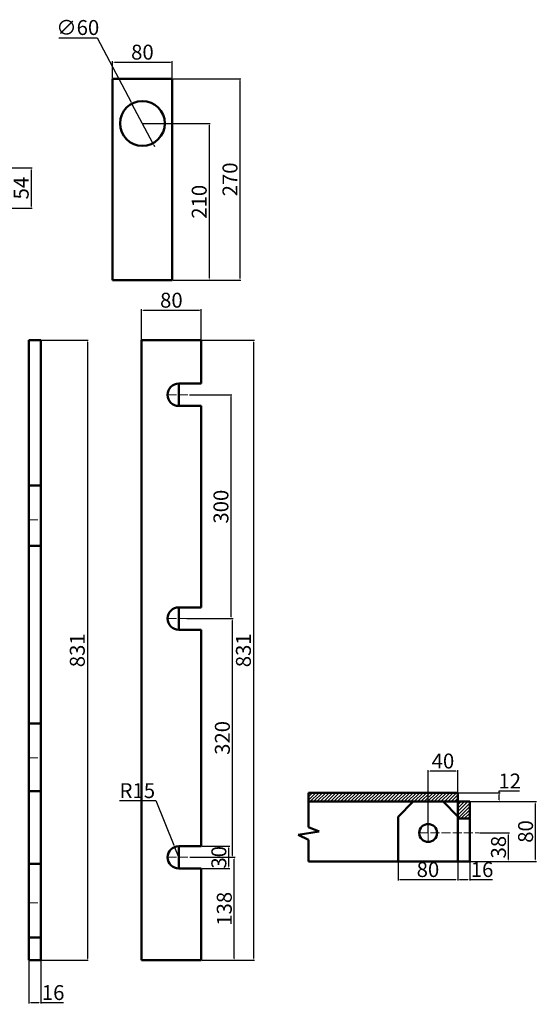
# Model space of a CAD drawing. Units: millimetres. Extents: x 1372 to 2780, y 1459 to 2779.
# Tile 2 of 2: x 2087 to 2780, y 1459 to 2779. Entities that reach past the tile are written whole.
import ezdxf

# ---------------------------------------------------------------- set-up
doc = ezdxf.new("R2010")
doc.units = ezdxf.units.MM
doc.linetypes.add('ACAD_ISO02W100', pattern=[15, 12, -3])
for name, color, linetype, lineweight in [('M-CNTR', 1, 'ACAD_ISO02W100', 18), ('M-DIMS', 2, 'Continuous', 25), ('M-HATC', 8, 'Continuous', 18), ('M-OUTL', 7, 'Continuous', 50)]:
    doc.layers.add(name, color=color, linetype=linetype, lineweight=lineweight)
doc.styles.get("Standard").update_dxf_attribs({"font": 'arial.ttf'})
doc.dimstyles.new('ISO-25', dxfattribs={"dimtxt": 20, "dimasz": 2.5, "dimexe": 1.25, "dimexo": 0.625, "dimtad": 1, "dimtoh": 1, "dimdec": 0, "dimtxsty": 'Standard', "dimcen": 2.5, "dimadec": 0, "dimazin": 0, "dimtfac": 1, "dimtdec": 0, "dimtmove": 0, "dimatfit": 3, "dimfxl": 1, "dimarcsym": 0})

# ---------------------------------------------------------------- blocks, each defined once
blk = doc.blocks.new('*D12')
at = {"layer": 'Defpoints', "color": 0, "transparency": 16777216}
for p in [(2099, 1518), (2115, 1518), (2115, 1461.3)]:
    blk.add_point(p, dxfattribs=at)
at = {"layer": 'M-DIMS', "color": 0, "lineweight": -2, "transparency": 16777216}
for p, q in [((2099, 1517.4), (2099, 1460)), ((2115, 1517.4), (2115, 1460)), ((2101.5, 1461.3), (2112.5, 1461.3)), ((2115, 1461.3), (2145.5, 1461.3))]:
    blk.add_line(p, q, dxfattribs=at)
at = {"layer": 'M-DIMS', "color": 0, "transparency": 16777216}
for points in [[(2101.5, 1461.7), (2101.5, 1460.8), (2099, 1461.3)], [(2112.5, 1461.7), (2112.5, 1460.8), (2115, 1461.3)]]:
    blk.add_solid(points, dxfattribs=at)
at = {"layer": 'M-DIMS', "color": 0, "transparency": 16777216, "insert": (2131.5, 1472.1), "char_height": 20, "attachment_point": 5}
blk.add_mtext('16', dxfattribs=at)
blk = doc.blocks.new('*D13')
at = {"layer": 'Defpoints', "color": 0, "transparency": 16777216}
for p in [(2115, 2349), (2115, 1518), (2177.4, 1518)]:
    blk.add_point(p, dxfattribs=at)
at = {"layer": 'M-DIMS', "color": 0, "lineweight": -2, "transparency": 16777216}
for p, q in [((2115.7, 2349), (2178.6, 2349)), ((2177.4, 2346.5), (2177.4, 1520.5)), ((2115.7, 1518), (2178.6, 1518))]:
    blk.add_line(p, q, dxfattribs=at)
at = {"layer": 'M-DIMS', "color": 0, "transparency": 16777216}
for points in [[(2176.9, 2346.5), (2177.8, 2346.5), (2177.4, 2349)], [(2176.9, 1520.5), (2177.8, 1520.5), (2177.4, 1518)]]:
    blk.add_solid(points, dxfattribs=at)
at = {"layer": 'M-DIMS', "color": 0, "transparency": 16777216, "insert": (2166.5, 1933.5), "char_height": 20, "attachment_point": 5, "rotation": 90}
blk.add_mtext('831', dxfattribs=at)
blk = doc.blocks.new('*D14')
at = {"layer": 'Defpoints', "color": 0, "transparency": 16777216}
for p in [(2329.9, 2349), (2329.9, 1518), (2399.9, 1518)]:
    blk.add_point(p, dxfattribs=at)
at = {"layer": 'M-DIMS', "color": 0, "lineweight": -2, "transparency": 16777216}
for p, q in [((2330.5, 2349), (2401.1, 2349)), ((2399.9, 2346.5), (2399.9, 1520.5)), ((2330.5, 1518), (2401.1, 1518))]:
    blk.add_line(p, q, dxfattribs=at)
at = {"layer": 'M-DIMS', "color": 0, "transparency": 16777216}
for points in [[(2399.5, 2346.5), (2400.3, 2346.5), (2399.9, 2349)], [(2399.5, 1520.5), (2400.3, 1520.5), (2399.9, 1518)]]:
    blk.add_solid(points, dxfattribs=at)
at = {"layer": 'M-DIMS', "color": 0, "transparency": 16777216, "insert": (2389, 1933.5), "char_height": 20, "attachment_point": 5, "rotation": 90}
blk.add_mtext('831', dxfattribs=at)
blk = doc.blocks.new('*D15')
at = {"layer": 'Defpoints', "color": 0, "transparency": 16777216}
for p in [(2329.9, 1671), (2366.9, 1671), (2329.9, 1641)]:
    blk.add_point(p, dxfattribs=at)
at = {"layer": 'M-DIMS', "color": 0, "lineweight": -2, "transparency": 16777216}
for p, q in [((2330.5, 1671), (2368.2, 1671)), ((2366.9, 1643.5), (2366.9, 1668.5)), ((2330.5, 1641), (2368.2, 1641))]:
    blk.add_line(p, q, dxfattribs=at)
at = {"layer": 'M-DIMS', "color": 0, "transparency": 16777216}
for points in [[(2366.5, 1668.5), (2367.3, 1668.5), (2366.9, 1671)], [(2366.5, 1643.5), (2367.3, 1643.5), (2366.9, 1641)]]:
    blk.add_solid(points, dxfattribs=at)
at = {"layer": 'M-DIMS', "color": 0, "transparency": 16777216, "insert": (2356.1, 1656), "char_height": 20, "attachment_point": 5, "rotation": 90}
blk.add_mtext('30', dxfattribs=at)
blk = doc.blocks.new('*D16')
at = {"layer": 'Defpoints', "color": 0, "transparency": 16777216}
for p in [(2294.2, 1669.9), (2299.9, 1656)]:
    blk.add_point(p, dxfattribs=at)
at = {"layer": 'M-DIMS', "color": 0, "lineweight": -2, "transparency": 16777216}
for p, q in [((2220.3, 1732), (2268.9, 1732)), ((2268.9, 1732), (2293.3, 1672.2)), ((2299.9, 1656), (2294.2, 1669.9))]:
    blk.add_line(p, q, dxfattribs=at)
at = {"layer": 'M-DIMS', "color": 0, "transparency": 16777216}
blk.add_solid([(2293.6, 1672.4), (2292.9, 1672), (2294.2, 1669.9)], dxfattribs=at)
at = {"layer": 'M-DIMS', "color": 0, "transparency": 16777216, "insert": (2244.3, 1742.8), "char_height": 20, "attachment_point": 5}
blk.add_mtext('R15', dxfattribs=at)
blk = doc.blocks.new('*D17')
at = {"layer": 'Defpoints', "color": 0, "transparency": 16777216}
for p in [(2314, 1656), (2374.2, 1656), (2329.9, 1518)]:
    blk.add_point(p, dxfattribs=at)
at = {"layer": 'M-DIMS', "color": 0, "lineweight": -2, "transparency": 16777216}
for p, q in [((2314.6, 1656), (2375.5, 1656)), ((2374.2, 1520.5), (2374.2, 1653.5)), ((2330.5, 1518), (2375.5, 1518))]:
    blk.add_line(p, q, dxfattribs=at)
at = {"layer": 'M-DIMS', "color": 0, "transparency": 16777216}
for points in [[(2373.8, 1653.5), (2374.6, 1653.5), (2374.2, 1656)], [(2373.8, 1520.5), (2374.6, 1520.5), (2374.2, 1518)]]:
    blk.add_solid(points, dxfattribs=at)
at = {"layer": 'M-DIMS', "color": 0, "transparency": 16777216, "insert": (2363.4, 1587), "char_height": 20, "attachment_point": 5, "rotation": 90}
blk.add_mtext('138', dxfattribs=at)
blk = doc.blocks.new('*D18')
at = {"layer": 'Defpoints', "color": 0, "transparency": 16777216}
for p in [(2309.9, 1976), (2371.7, 1976), (2314, 1656)]:
    blk.add_point(p, dxfattribs=at)
at = {"layer": 'M-DIMS', "color": 0, "lineweight": -2, "transparency": 16777216}
for p, q in [((2310.5, 1976), (2372.9, 1976)), ((2371.7, 1658.5), (2371.7, 1973.5)), ((2314.6, 1656), (2372.9, 1656))]:
    blk.add_line(p, q, dxfattribs=at)
at = {"layer": 'M-DIMS', "color": 0, "transparency": 16777216}
for points in [[(2371.2, 1973.5), (2372.1, 1973.5), (2371.7, 1976)], [(2371.2, 1658.5), (2372.1, 1658.5), (2371.7, 1656)]]:
    blk.add_solid(points, dxfattribs=at)
at = {"layer": 'M-DIMS', "color": 0, "transparency": 16777216, "insert": (2360.8, 1816), "char_height": 20, "attachment_point": 5, "rotation": 90}
blk.add_mtext('320', dxfattribs=at)
blk = doc.blocks.new('*D19')
at = {"layer": 'Defpoints', "color": 0, "transparency": 16777216}
for p in [(2313.5, 2276), (2369.8, 2276), (2309.9, 1976)]:
    blk.add_point(p, dxfattribs=at)
at = {"layer": 'M-DIMS', "color": 0, "lineweight": -2, "transparency": 16777216}
for p, q in [((2314.2, 2276), (2371, 2276)), ((2369.8, 1978.5), (2369.8, 2273.5)), ((2310.5, 1976), (2371, 1976))]:
    blk.add_line(p, q, dxfattribs=at)
at = {"layer": 'M-DIMS', "color": 0, "transparency": 16777216}
for points in [[(2369.4, 2273.5), (2370.2, 2273.5), (2369.8, 2276)], [(2369.4, 1978.5), (2370.2, 1978.5), (2369.8, 1976)]]:
    blk.add_solid(points, dxfattribs=at)
at = {"layer": 'M-DIMS', "color": 0, "transparency": 16777216, "insert": (2358.9, 2126), "char_height": 20, "attachment_point": 5, "rotation": 90}
blk.add_mtext('300', dxfattribs=at)
blk = doc.blocks.new('*D20')
at = {"layer": 'Defpoints', "color": 0, "transparency": 16777216}
for p in [(2329.9, 2389.3), (2249.9, 2349), (2329.9, 2349)]:
    blk.add_point(p, dxfattribs=at)
at = {"layer": 'M-DIMS', "color": 0, "lineweight": -2, "transparency": 16777216}
for p, q in [((2249.9, 2349.6), (2249.9, 2390.6)), ((2252.4, 2389.3), (2327.4, 2389.3)), ((2329.9, 2349.6), (2329.9, 2390.6))]:
    blk.add_line(p, q, dxfattribs=at)
at = {"layer": 'M-DIMS', "color": 0, "transparency": 16777216}
for points in [[(2252.4, 2389.7), (2252.4, 2388.9), (2249.9, 2389.3)], [(2327.4, 2389.7), (2327.4, 2388.9), (2329.9, 2389.3)]]:
    blk.add_solid(points, dxfattribs=at)
at = {"layer": 'M-DIMS', "color": 0, "transparency": 16777216, "insert": (2289.9, 2400.2), "char_height": 20, "attachment_point": 5}
blk.add_mtext('80', dxfattribs=at)
blk = doc.blocks.new('*D21')
at = {"layer": 'Defpoints', "color": 0, "transparency": 16777216}
for p in [(2593.6, 1650.6), (2673.6, 1650.6), (2673.6, 1626.2)]:
    blk.add_point(p, dxfattribs=at)
at = {"layer": 'M-DIMS', "color": 0, "lineweight": -2, "transparency": 16777216}
for p, q in [((2593.6, 1649.9), (2593.6, 1625)), ((2673.6, 1649.9), (2673.6, 1625)), ((2596.1, 1626.2), (2671.1, 1626.2))]:
    blk.add_line(p, q, dxfattribs=at)
at = {"layer": 'M-DIMS', "color": 0, "transparency": 16777216}
for points in [[(2596.1, 1626.6), (2596.1, 1625.8), (2593.6, 1626.2)], [(2671.1, 1626.6), (2671.1, 1625.8), (2673.6, 1626.2)]]:
    blk.add_solid(points, dxfattribs=at)
at = {"layer": 'M-DIMS', "color": 0, "transparency": 16777216, "insert": (2633.6, 1637), "char_height": 20, "attachment_point": 5}
blk.add_mtext('80', dxfattribs=at)
blk = doc.blocks.new('*D22')
at = {"layer": 'Defpoints', "color": 0, "transparency": 16777216}
for p in [(2673.6, 1650.6), (2689.6, 1650.6), (2689.6, 1626.2)]:
    blk.add_point(p, dxfattribs=at)
at = {"layer": 'M-DIMS', "color": 0, "lineweight": -2, "transparency": 16777216}
for p, q in [((2673.6, 1649.9), (2673.6, 1625)), ((2689.6, 1649.9), (2689.6, 1625)), ((2676.1, 1626.2), (2687.1, 1626.2)), ((2689.6, 1626.2), (2720.1, 1626.2))]:
    blk.add_line(p, q, dxfattribs=at)
at = {"layer": 'M-DIMS', "color": 0, "transparency": 16777216}
for points in [[(2676.1, 1626.6), (2676.1, 1625.8), (2673.6, 1626.2)], [(2687.1, 1626.6), (2687.1, 1625.8), (2689.6, 1626.2)]]:
    blk.add_solid(points, dxfattribs=at)
at = {"layer": 'M-DIMS', "color": 0, "transparency": 16777216, "insert": (2706.1, 1637), "char_height": 20, "attachment_point": 5}
blk.add_mtext('16', dxfattribs=at)
blk = doc.blocks.new('*D23')
at = {"layer": 'Defpoints', "color": 0, "transparency": 16777216}
for p in [(2701.9, 1688.6), (2741.5, 1688.6), (2689.6, 1650.6)]:
    blk.add_point(p, dxfattribs=at)
at = {"layer": 'M-DIMS', "color": 0, "lineweight": -2, "transparency": 16777216}
for p, q in [((2702.6, 1688.6), (2742.8, 1688.6)), ((2741.5, 1653.1), (2741.5, 1686.1)), ((2690.2, 1650.6), (2742.8, 1650.6))]:
    blk.add_line(p, q, dxfattribs=at)
at = {"layer": 'M-DIMS', "color": 0, "transparency": 16777216}
for points in [[(2741.1, 1686.1), (2741.9, 1686.1), (2741.5, 1688.6)], [(2741.1, 1653.1), (2741.9, 1653.1), (2741.5, 1650.6)]]:
    blk.add_solid(points, dxfattribs=at)
at = {"layer": 'M-DIMS', "color": 0, "transparency": 16777216, "insert": (2730.7, 1669.6), "char_height": 20, "attachment_point": 5, "rotation": 90}
blk.add_mtext('38', dxfattribs=at)
blk = doc.blocks.new('*D24')
at = {"layer": 'Defpoints', "color": 0, "transparency": 16777216}
for p in [(2689.6, 1730.6), (2777.8, 1730.6), (2689.6, 1650.6)]:
    blk.add_point(p, dxfattribs=at)
at = {"layer": 'M-DIMS', "color": 0, "lineweight": -2, "transparency": 16777216}
for p, q in [((2690.2, 1730.6), (2779.1, 1730.6)), ((2777.8, 1653.1), (2777.8, 1728.1)), ((2690.2, 1650.6), (2779.1, 1650.6))]:
    blk.add_line(p, q, dxfattribs=at)
at = {"layer": 'M-DIMS', "color": 0, "transparency": 16777216}
for points in [[(2777.4, 1728.1), (2778.2, 1728.1), (2777.8, 1730.6)], [(2777.4, 1653.1), (2778.2, 1653.1), (2777.8, 1650.6)]]:
    blk.add_solid(points, dxfattribs=at)
at = {"layer": 'M-DIMS', "color": 0, "transparency": 16777216, "insert": (2767, 1690.6), "char_height": 20, "attachment_point": 5, "rotation": 90}
blk.add_mtext('80', dxfattribs=at)
blk = doc.blocks.new('*D25')
at = {"layer": 'Defpoints', "color": 0, "transparency": 16777216}
for p in [(2673.6, 1742.6), (2729.2, 1742.6), (2673.6, 1730.6)]:
    blk.add_point(p, dxfattribs=at)
at = {"layer": 'M-DIMS', "color": 0, "lineweight": -2, "transparency": 16777216}
for p, q in [((2674.2, 1742.6), (2730.4, 1742.6)), ((2729.2, 1742.6), (2729.2, 1745.1)), ((2729.2, 1745.1), (2756.3, 1745.1)), ((2674.2, 1730.6), (2730.4, 1730.6)), ((2729.2, 1733.1), (2729.2, 1740.1))]:
    blk.add_line(p, q, dxfattribs=at)
at = {"layer": 'M-DIMS', "color": 0, "transparency": 16777216}
for points in [[(2728.7, 1740.1), (2729.6, 1740.1), (2729.2, 1742.6)], [(2728.7, 1733.1), (2729.6, 1733.1), (2729.2, 1730.6)]]:
    blk.add_solid(points, dxfattribs=at)
at = {"layer": 'M-DIMS', "color": 0, "transparency": 16777216, "insert": (2743.1, 1755.7), "char_height": 20, "attachment_point": 5}
blk.add_mtext('12', dxfattribs=at)
blk = doc.blocks.new('*D26')
at = {"layer": 'Defpoints', "color": 0, "transparency": 16777216}
for p in [(2633.9, 1771.6), (2673.6, 1730.6), (2633.9, 1688.6)]:
    blk.add_point(p, dxfattribs=at)
at = {"layer": 'M-DIMS', "color": 0, "lineweight": -2, "transparency": 16777216}
for p, q in [((2633.9, 1689.2), (2633.9, 1772.9)), ((2671.1, 1771.6), (2636.4, 1771.6)), ((2673.6, 1731.2), (2673.6, 1772.9))]:
    blk.add_line(p, q, dxfattribs=at)
at = {"layer": 'M-DIMS', "color": 0, "transparency": 16777216}
for points in [[(2636.4, 1772), (2636.4, 1771.2), (2633.9, 1771.6)], [(2671.1, 1772), (2671.1, 1771.2), (2673.6, 1771.6)]]:
    blk.add_solid(points, dxfattribs=at)
at = {"layer": 'M-DIMS', "color": 0, "transparency": 16777216, "insert": (2653.7, 1782.5), "char_height": 20, "attachment_point": 5}
blk.add_mtext('40', dxfattribs=at)
blk = doc.blocks.new('*D49')
at = {"layer": 'Defpoints', "color": 0, "transparency": 16777216}
for p in [(2008, 2580), (2022, 2526), (2102.1, 2526)]:
    blk.add_point(p, dxfattribs=at)
at = {"layer": 'M-DIMS', "color": 0, "lineweight": -2, "transparency": 16777216}
for p, q in [((2008.6, 2580), (2103.3, 2580)), ((2102.1, 2577.5), (2102.1, 2528.5)), ((2022.6, 2526), (2103.3, 2526))]:
    blk.add_line(p, q, dxfattribs=at)
at = {"layer": 'M-DIMS', "color": 0, "transparency": 16777216}
for points in [[(2101.7, 2577.5), (2102.5, 2577.5), (2102.1, 2580)], [(2101.7, 2528.5), (2102.5, 2528.5), (2102.1, 2526)]]:
    blk.add_solid(points, dxfattribs=at)
at = {"layer": 'M-DIMS', "color": 0, "transparency": 16777216, "insert": (2091.3, 2553), "char_height": 20, "attachment_point": 5, "rotation": 90}
blk.add_mtext('54', dxfattribs=at)
blk = doc.blocks.new('*D52')
at = {"layer": 'Defpoints', "color": 0, "transparency": 16777216}
for p in [(2291.1, 2721.9), (2211.1, 2699.7), (2291.1, 2699.7)]:
    blk.add_point(p, dxfattribs=at)
at = {"layer": 'M-DIMS', "color": 0, "lineweight": -2, "transparency": 16777216}
for p, q in [((2211.1, 2700.3), (2211.1, 2723.1)), ((2213.6, 2721.9), (2288.6, 2721.9)), ((2291.1, 2700.3), (2291.1, 2723.1))]:
    blk.add_line(p, q, dxfattribs=at)
at = {"layer": 'M-DIMS', "color": 0, "transparency": 16777216}
for points in [[(2213.6, 2722.3), (2213.6, 2721.5), (2211.1, 2721.9)], [(2288.6, 2722.3), (2288.6, 2721.5), (2291.1, 2721.9)]]:
    blk.add_solid(points, dxfattribs=at)
at = {"layer": 'M-DIMS', "color": 0, "transparency": 16777216, "insert": (2251.1, 2732.7), "char_height": 20, "attachment_point": 5}
blk.add_mtext('80', dxfattribs=at)
blk = doc.blocks.new('*D53')
at = {"layer": 'Defpoints', "color": 0, "transparency": 16777216}
for p in [(2291.1, 2699.7), (2291.1, 2429.7), (2381.8, 2429.7)]:
    blk.add_point(p, dxfattribs=at)
at = {"layer": 'M-DIMS', "color": 0, "lineweight": -2, "transparency": 16777216}
for p, q in [((2291.7, 2699.7), (2383.1, 2699.7)), ((2381.8, 2697.2), (2381.8, 2432.2)), ((2291.7, 2429.7), (2383.1, 2429.7))]:
    blk.add_line(p, q, dxfattribs=at)
at = {"layer": 'M-DIMS', "color": 0, "transparency": 16777216}
for points in [[(2381.4, 2697.2), (2382.2, 2697.2), (2381.8, 2699.7)], [(2381.4, 2432.2), (2382.2, 2432.2), (2381.8, 2429.7)]]:
    blk.add_solid(points, dxfattribs=at)
at = {"layer": 'M-DIMS', "color": 0, "transparency": 16777216, "insert": (2371, 2564.7), "char_height": 20, "attachment_point": 5, "rotation": 90}
blk.add_mtext('270', dxfattribs=at)
blk = doc.blocks.new('*D54')
at = {"layer": 'Defpoints', "color": 0, "transparency": 16777216}
for p in [(2251.1, 2639.7), (2291.1, 2429.7), (2340.6, 2429.7)]:
    blk.add_point(p, dxfattribs=at)
at = {"layer": 'M-DIMS', "color": 0, "lineweight": -2, "transparency": 16777216}
for p, q in [((2251.7, 2639.7), (2341.9, 2639.7)), ((2340.6, 2637.2), (2340.6, 2432.2)), ((2291.7, 2429.7), (2341.9, 2429.7))]:
    blk.add_line(p, q, dxfattribs=at)
at = {"layer": 'M-DIMS', "color": 0, "transparency": 16777216}
for points in [[(2340.2, 2637.2), (2341, 2637.2), (2340.6, 2639.7)], [(2340.2, 2432.2), (2341, 2432.2), (2340.6, 2429.7)]]:
    blk.add_solid(points, dxfattribs=at)
at = {"layer": 'M-DIMS', "color": 0, "transparency": 16777216, "insert": (2329.8, 2534.7), "char_height": 20, "attachment_point": 5, "rotation": 90}
blk.add_mtext('210', dxfattribs=at)
blk = doc.blocks.new('*D55')
at = {"layer": 'Defpoints', "color": 0, "transparency": 16777216}
for p in [(2237, 2666.2), (2265.2, 2613.2)]:
    blk.add_point(p, dxfattribs=at)
at = {"layer": 'M-DIMS', "color": 0, "lineweight": -2, "transparency": 16777216}
for p, q in [((2139.3, 2754.3), (2190.3, 2754.3)), ((2190.3, 2754.3), (2235.9, 2668.4)), ((2265.2, 2613.2), (2237, 2666.2)), ((2266.3, 2611), (2267.5, 2608.8))]:
    blk.add_line(p, q, dxfattribs=at)
at = {"layer": 'M-DIMS', "color": 0, "transparency": 16777216}
for points in [[(2236.2, 2668.6), (2235.5, 2668.2), (2237, 2666.2)], [(2266.7, 2611.2), (2266, 2610.8), (2265.2, 2613.2)]]:
    blk.add_solid(points, dxfattribs=at)
at = {"layer": 'M-DIMS', "color": 0, "transparency": 16777216, "insert": (2164.5, 2765.7), "char_height": 20, "attachment_point": 5}
blk.add_mtext('∅60', dxfattribs=at)

msp = doc.modelspace()

# ---------------------------------------------------------------- hatches: boundary and pattern name
at = {"layer": 'M-HATC'}
h = msp.add_hatch(dxfattribs=at)
h.set_pattern_fill('ANSI31', color=256)
h.paths.add_polyline_path([(2673.6, 1742.6), (2473.6, 1742.6), (2473.6, 1730.6), (2673.6, 1730.6)])
h.paths.add_polyline_path([(2689.6, 1730.6), (2673.6, 1730.6), (2673.6, 1707.9), (2689.6, 1707.9)])

# ---------------------------------------------------------------- linework, layer by layer
at = {"layer": 'M-CNTR'}
for p, q in [((2284.9, 2276), (2342.2, 2276)), ((2099, 2108.2), (2115, 2108.2)), ((2284.9, 1976), (2334.9, 1976)), ((2099, 1789.3), (2115, 1789.3)), ((2633.9, 1676.6), (2633.9, 1715.7)), ((2621.9, 1688.6), (2701.9, 1688.6)), ((2284.9, 1656), (2343.1, 1656)), ((2099, 1595), (2115, 1595))]:
    msp.add_line(p, q, dxfattribs=at)
at = {"layer": 'M-OUTL'}
for p, q in [((2211.1, 2699.7), (2211.1, 2429.7)), ((2291.1, 2699.7), (2211.1, 2699.7)), ((2291.1, 2429.7), (2291.1, 2699.7)), ((2211.1, 2429.7), (2291.1, 2429.7)), ((2099, 1518), (2099, 2349)), ((2099, 2349), (2115, 2349)), ((2115, 2349), (2115, 1518)), ((2249.9, 2349), (2249.9, 1518)), ((2249.9, 2349), (2329.9, 2349)), ((2329.9, 2349), (2329.9, 2291)), ((2299.9, 2291), (2329.9, 2291)), ((2299.9, 2291), (2299.9, 2261)), ((2299.9, 2261), (2329.9, 2261)), ((2329.9, 1991), (2329.9, 2261)), ((2099, 2154.6), (2115, 2154.6)), ((2115, 2073.5), (2099, 2073.5)), ((2299.9, 1991), (2329.9, 1991)), ((2299.9, 1991), (2299.9, 1961)), ((2299.9, 1961), (2329.9, 1961)), ((2329.9, 1671), (2329.9, 1961)), ((2329.9, 1961), (2329.9, 1919.9)), ((2099, 1835.3), (2115, 1835.3)), ((2115, 1744.5), (2099, 1744.5)), ((2473.6, 1730.6), (2473.6, 1742.6)), ((2473.6, 1742.6), (2673.6, 1742.6)), ((2673.6, 1742.6), (2673.6, 1730.6)), ((2673.6, 1730.6), (2473.6, 1730.6)), ((2473.6, 1730.6), (2473.6, 1700.8)), ((2593.6, 1730.6), (2613.6, 1730.6)), ((2613.6, 1730.6), (2593.6, 1710.1)), ((2654.1, 1730.6), (2673.6, 1710.6)), ((2689.6, 1730.6), (2673.6, 1730.6)), ((2673.6, 1730.6), (2673.6, 1650.6)), ((2689.6, 1650.6), (2689.6, 1730.6)), ((2593.6, 1650.6), (2593.6, 1710.1)), ((2673.6, 1707.9), (2689.6, 1707.9)), ((2459.6, 1686.3), (2488.1, 1690.5)), ((2473.6, 1700.8), (2473.6, 1696.2)), ((2488.1, 1690.5), (2473.6, 1696.2)), ((2473.6, 1679.6), (2459.6, 1686.3)), ((2473.6, 1667.7), (2473.6, 1679.6)), ((2593.6, 1650.6), (2593.6, 1688.6)), ((2299.9, 1671), (2329.9, 1671)), ((2299.9, 1671), (2299.9, 1641)), ((2473.6, 1667.7), (2473.6, 1650.6)), ((2489.6, 1650.6), (2473.6, 1650.6)), ((2489.6, 1650.6), (2689.6, 1650.6)), ((2673.6, 1650.6), (2593.6, 1650.6)), ((2099, 1647.1), (2115, 1647.1)), ((2299.9, 1641), (2329.9, 1641)), ((2329.9, 1518), (2329.9, 1641)), ((2115, 1548.4), (2099, 1548.4)), ((2115, 1518), (2099, 1518)), ((2249.9, 1518), (2329.9, 1518))]:
    msp.add_line(p, q, dxfattribs=at)
for centre, radius in [((2251.1, 2639.7), 30), ((2633.9, 1688.6), 12)]:
    msp.add_circle(centre, radius, dxfattribs=at)
for centre in [(2299.9, 2276), (2299.9, 1976), (2299.9, 1656)]:
    msp.add_arc(centre, 15, 90, 270, dxfattribs=at)

# ---------------------------------------------------------------- dimensions: what is measured, and where the dimension line sits
at = {"layer": 'M-DIMS'}
dim = msp.add_diameter_dim_2p(p1=(2265.2, 2613.2), p2=(2237, 2666.2), dimstyle='ISO-25', override={"dimclrd": 0, "dimclre": 0, "dimclrt": 0}, dxfattribs=at)
dim.commit()
dim.dimension.update_dxf_attribs({"geometry": '*D55', "text_midpoint": (2164.5, 2754.3), "dimtype": 163})
for base, p1, p2, picture, middle in [((2291.1, 2721.9), (2211.1, 2699.7), (2291.1, 2699.7), '*D52', (2251.1, 2732.7)), ((2329.9, 2389.3), (2249.9, 2349), (2329.9, 2349), '*D20', (2289.9, 2400.2)), ((2633.9, 1771.6), (2673.6, 1730.6), (2633.9, 1688.6), '*D26', (2653.7, 1782.5)), ((2673.6, 1626.2), (2593.6, 1650.6), (2673.6, 1650.6), '*D21', (2633.6, 1637)), ((2689.6, 1626.2), (2673.6, 1650.6), (2689.6, 1650.6), '*D22', (2706.1, 1637)), ((2115, 1461.3), (2099, 1518), (2115, 1518), '*D12', (2131.5, 1472.1))]:
    dim = msp.add_linear_dim(base=base, p1=p1, p2=p2, dimstyle='ISO-25', override={"dimclrd": 0, "dimclre": 0, "dimclrt": 0}, dxfattribs=at)
    dim.commit()
    dim.dimension.update_dxf_attribs({"geometry": picture, "text_midpoint": middle})
for base, p1, p2, picture, middle in [((2381.8, 2429.7), (2291.1, 2699.7), (2291.1, 2429.7), '*D53', (2371, 2564.7)), ((2340.6, 2429.7), (2251.1, 2639.7), (2291.1, 2429.7), '*D54', (2329.8, 2534.7)), ((2102.1, 2526), (2008, 2580), (2022, 2526), '*D49', (2091.3, 2553)), ((2177.4, 1518), (2115, 2349), (2115, 1518), '*D13', (2166.5, 1933.5)), ((2399.9, 1518), (2329.9, 2349), (2329.9, 1518), '*D14', (2389, 1933.5)), ((2369.8, 2276), (2309.9, 1976), (2313.5, 2276), '*D19', (2358.9, 2126)), ((2371.7, 1976), (2314, 1656), (2309.9, 1976), '*D18', (2360.8, 1816)), ((2729.2, 1742.6), (2673.6, 1730.6), (2673.6, 1742.6), '*D25', (2743.1, 1755.7)), ((2777.8, 1730.6), (2689.6, 1650.6), (2689.6, 1730.6), '*D24', (2767, 1690.6)), ((2741.5, 1688.6), (2689.6, 1650.6), (2701.9, 1688.6), '*D23', (2730.7, 1669.6)), ((2366.9, 1671), (2329.9, 1641), (2329.9, 1671), '*D15', (2356.1, 1656)), ((2374.2, 1656), (2329.9, 1518), (2314, 1656), '*D17', (2363.4, 1587))]:
    dim = msp.add_linear_dim(base=base, p1=p1, p2=p2, angle=90, dimstyle='ISO-25', override={"dimclrd": 0, "dimclre": 0, "dimclrt": 0}, dxfattribs=at)
    dim.commit()
    dim.dimension.update_dxf_attribs({"geometry": picture, "text_midpoint": middle})
dim = msp.add_radius_dim(center=(2299.9, 1656), mpoint=(2294.2, 1669.9), dimstyle='ISO-25', override={"dimclrd": 0, "dimclre": 0, "dimclrt": 0}, dxfattribs=at)
dim.commit()
dim.dimension.update_dxf_attribs({"geometry": '*D16', "text_midpoint": (2244.3, 1732), "dimtype": 164})

doc.saveas('drawing.dxf')
